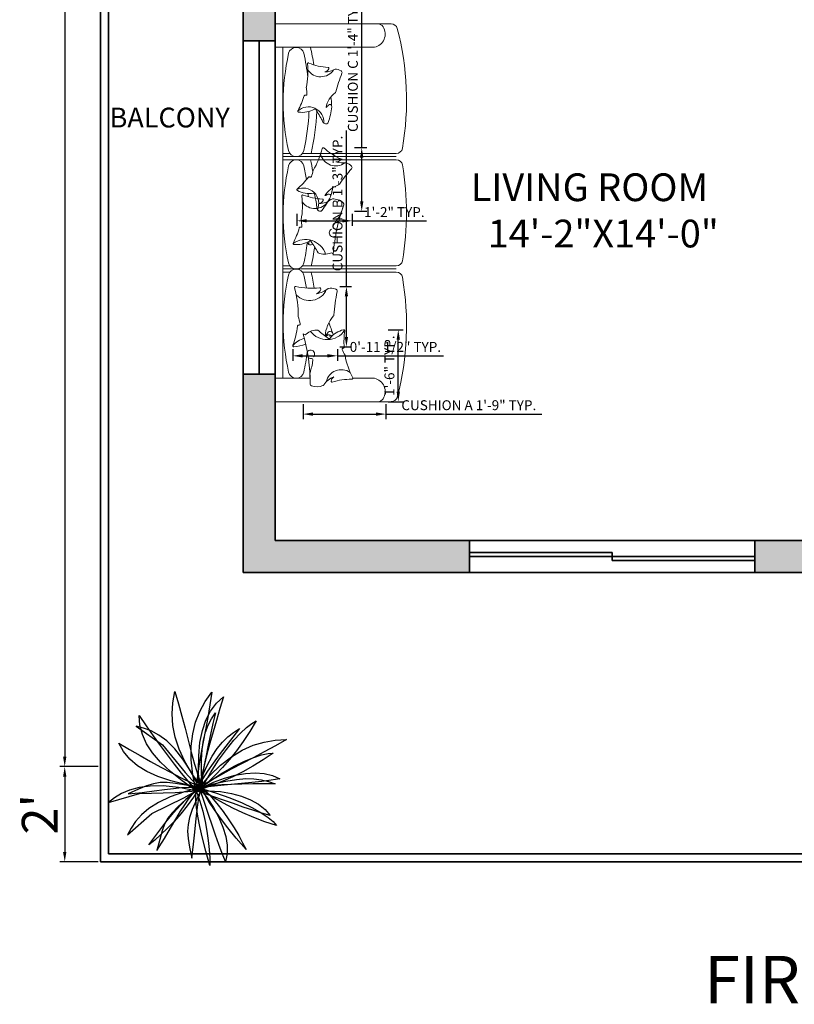
# Model space of a CAD drawing. Units: inches. Extents: x 1566 to 2546, y 1087 to 2705.
# Tile 12 of 27: x 2042 to 2237, y 1100 to 1349. Entities that reach past the tile are written whole.
import ezdxf

# ---------------------------------------------------------------- set-up
doc = ezdxf.new("R2010")
doc.units = ezdxf.units.IN
for name, color, linetype, lineweight in [('A-ANNO-DIMS', 2, 'Continuous', 18), ('A-AREA-IDEN', 7, 'Continuous', 18), ('A-FURN', 8, 'Continuous', 18), ('A-WALL', 7, 'Continuous', 35), ('A-WALL-PATT', 8, 'Continuous', 13), ('L-PLNT', 94, 'Continuous', 18)]:
    doc.layers.add(name, color=color, linetype=linetype, lineweight=lineweight)
doc.layers.add('DIENHOA', color=3, linetype='Continuous')
doc.styles.get("Standard").update_dxf_attribs({"font": 'arial.ttf'})
doc.dimstyles.new('ISO-25', dxfattribs={"dimtxt": 2.5, "dimasz": 2.5, "dimexe": 1.25, "dimexo": 0.625, "dimtad": 1, "dimtxsty": 'Standard', "dimcen": 2.5, "dimadec": 0, "dimazin": 0, "dimtfac": 1, "dimtmove": 0, "dimatfit": 3, "dimfxl": 1, "dimarcsym": 0})

# ---------------------------------------------------------------- blocks, each defined once
blk = doc.blocks.new('*D3')
at = {"layer": 'A-ANNO-DIMS', "color": 0, "lineweight": -2, "transparency": 16777216}
for p, q in [((2061.66, 1784.43), (2052.02, 1784.43)), ((2053.27, 1781.93), (2053.27, 1162.93)), ((2061.66, 1160.43), (2052.02, 1160.43))]:
    blk.add_line(p, q, dxfattribs=at)
at = {"layer": 'A-ANNO-DIMS', "color": 0, "transparency": 16777216}
for points in [[(2052.85, 1781.93), (2053.69, 1781.93), (2053.27, 1784.43)], [(2052.85, 1162.93), (2053.69, 1162.93), (2053.27, 1160.43)]]:
    blk.add_solid(points, dxfattribs=at)
at = {"layer": 'Defpoints', "color": 0, "transparency": 16777216}
for p in [(2062.29, 1784.43), (2053.27, 1160.43), (2062.29, 1160.43)]:
    blk.add_point(p, dxfattribs=at)
at = {"layer": 'A-ANNO-DIMS', "color": 0, "transparency": 16777216, "insert": (2048.05, 1472.43), "char_height": 9, "attachment_point": 5, "rotation": 90}
blk.add_mtext("52'", dxfattribs=at)
blk = doc.blocks.new('*D4')
at = {"layer": 'A-ANNO-DIMS', "color": 0, "lineweight": -2, "transparency": 16777216}
for p, q in [((2061.66, 1160.43), (2052.02, 1160.43)), ((2053.27, 1157.93), (2053.27, 1138.93)), ((2061.66, 1136.43), (2052.02, 1136.43))]:
    blk.add_line(p, q, dxfattribs=at)
at = {"layer": 'A-ANNO-DIMS', "color": 0, "transparency": 16777216}
for points in [[(2052.85, 1157.93), (2053.69, 1157.93), (2053.27, 1160.43)], [(2052.85, 1138.93), (2053.69, 1138.93), (2053.27, 1136.43)]]:
    blk.add_solid(points, dxfattribs=at)
at = {"layer": 'Defpoints', "color": 0, "transparency": 16777216}
for p in [(2062.29, 1160.43), (2053.27, 1136.43), (2062.29, 1136.43)]:
    blk.add_point(p, dxfattribs=at)
at = {"layer": 'A-ANNO-DIMS', "color": 0, "transparency": 16777216, "insert": (2048.13, 1148.43), "char_height": 9, "attachment_point": 5, "rotation": 90}
blk.add_mtext("2'", dxfattribs=at)
blk = doc.blocks.new('Cay03_mb')
at = {"layer": 'DIENHOA'}
for p, q in [((118.6, 555.3), (166.2, 599.1)), ((166.2, 599.1), (142.2, 519.4)), ((79.5, 503.7), (118.6, 555.3)), ((48.6, 443.6), (79.5, 503.7)), ((142.2, 519.4), (119, 441.7)), ((-365.2, 390.3), (-414.4, 402.8)), ((-414.4, 402.8), (-240.2, 277.8)), ((25.5, 374.3), (48.6, 443.6)), ((119, 441.7), (96.7, 365.6)), ((-314.9, 371.3), (-365.2, 390.3)), ((-263.5, 343.5), (-314.9, 371.3)), ((-211.2, 304.6), (-263.5, 343.5)), ((9.9, 295.3), (25.5, 374.3)), ((96.7, 365.6), (75.6, 290.6)), ((-240.2, 277.8), (-88.4, 94.9)), ((-158, 252.3), (-211.2, 304.6)), ((1.6, 205.7), (9.9, 295.3)), ((75.6, 290.6), (55.7, 216.3)), ((290.6, 243.2), (363.4, 275.4)), ((363.4, 275.4), (436.8, 297.2)), ((436.8, 297.2), (511, 309.6)), ((511.8, 271.4), (437.6, 231.5)), ((511, 309.6), (585.9, 313.5)), ((585.9, 313.5), (511.8, 271.4)), ((-104.2, 184.4), (-158, 252.3)), ((0.2, 104.9), (1.6, 205.7)), ((55.7, 216.3), (37.3, 142.1)), ((147, 144.1), (218.5, 199.8)), ((218.5, 199.8), (290.6, 243.2)), ((437.6, 231.5), (363.7, 192.9)), ((-49.6, 98.5), (-104.2, 184.4)), ((37.3, 142.1), (20.5, 67.6)), ((75.9, 75.2), (147, 144.1)), ((290.2, 154.9), (217.4, 116.6)), ((363.7, 192.9), (290.2, 154.9)), ((-88.4, 94.9), (5.4, -7.8)), ((5.4, -7.8), (-49.6, 98.5)), ((5.4, -7.8), (0.2, 104.9)), ((5.4, -7.8), (75.9, 75.2)), ((20.5, 67.6), (5.4, -7.8)), ((145.5, 77.3), (74.7, 36.1)), ((217.4, 116.6), (145.5, 77.3)), ((-345, 5.4), (-399.6, -17.1)), ((-298.6, 20.1), (-345, 5.4)), ((-254.7, 27.4), (-298.6, 20.1)), ((-208, 27.8), (-254.7, 27.4)), ((-152.7, 21.7), (-208, 27.8)), ((-83.4, 9.7), (-152.7, 21.7)), ((5.4, -7.8), (-83.4, 9.7)), ((74.7, 36.1), (5.4, -7.8)), ((5.4, -7.8), (100.3, 18.4)), ((46.3, 0.9), (5.4, -7.8)), ((96.7, 7.5), (46.3, 0.9)), ((155, 12.2), (96.7, 7.5)), ((100.3, 18.4), (182.2, 37.2)), ((219.6, 15.4), (155, 12.2)), ((182.2, 37.2), (253, 48.9)), ((289, 17.4), (219.6, 15.4)), ((253, 48.9), (314.6, 54.1)), ((361.6, 18.5), (289, 17.4)), ((314.6, 54.1), (369.2, 53.3)), ((435.8, 18.9), (361.6, 18.5)), ((369.2, 53.3), (418.6, 46.8)), ((418.6, 46.8), (464.9, 35.2)), ((510, 19), (435.8, 18.9)), ((464.9, 35.2), (510, 19)), ((-399.6, -17.1), (-468, -47.9)), ((-468, -47.9), (-375.6, -37.8)), ((-375.6, -37.8), (-295.3, -27.9)), ((-295.3, -27.9), (-225.8, -18.9)), ((-225.8, -18.9), (-165.8, -11.3)), ((-165.8, -11.3), (-114, -5.7)), ((-114, -5.7), (-69, -2.9)), ((-79.8, -79.6), (-45.1, -46.3)), ((-69, -2.9), (-29.6, -3.4)), ((-45.1, -46.3), (-16.5, -22.4)), ((5.4, -7.8), (-33.2, -69.5)), ((-29.6, -3.4), (5.4, -7.8)), ((-16.5, -22.4), (5.4, -7.8)), ((5.4, -7.8), (56.8, -73.3)), ((25.9, -64.4), (5.4, -7.8)), ((5.4, -7.8), (112.8, -40.3)), ((53.5, -41.6), (5.4, -7.8)), ((47, -125.9), (25.9, -64.4)), ((107, -75.7), (53.5, -41.6)), ((112.8, -40.3), (207.5, -73.8)), ((-165.9, -174.1), (-120.2, -122.1)), ((-120.2, -122.1), (-79.8, -79.6)), ((-74.6, -127.3), (-117.8, -181.1)), ((-33.2, -69.5), (-74.6, -127.3)), ((68.7, -190.6), (47, -125.9)), ((56.8, -73.3), (100.4, -139.1)), ((165.5, -109.6), (107, -75.7)), ((228.7, -142.8), (165.5, -109.6)), ((207.5, -73.8), (289.5, -107.6)), ((289.5, -107.6), (359.3, -141.1)), ((-216.3, -235.6), (-165.9, -174.1)), ((-117.8, -181.1), (-162.1, -230.9)), ((90.8, -256.6), (68.7, -190.6)), ((100.4, -139.1), (135.9, -204.3)), ((296, -174.7), (228.7, -142.8)), ((367.1, -204.8), (296, -174.7)), ((359.3, -141.1), (416.9, -173.5)), ((416.9, -173.5), (462.6, -204.2)), ((-271, -306.6), (-216.3, -235.6)), ((-162.1, -230.9), (-206.3, -276.5)), ((113.1, -322.2), (90.8, -256.6)), ((135.9, -204.3), (162.8, -268.3)), ((441.6, -232.7), (367.1, -204.8)), ((518.9, -257.7), (441.6, -232.7)), ((462.6, -204.2), (496.5, -232.5)), ((496.5, -232.5), (518.9, -257.7)), ((-329.5, -387.1), (-271, -306.6)), ((-249.6, -317.8), (-291, -354.7)), ((-206.3, -276.5), (-249.6, -317.8)), ((135.4, -385.6), (113.1, -322.2)), ((162.8, -268.3), (181, -330.4)), ((-291, -354.7), (-329.5, -387.1)), ((157.6, -445), (135.4, -385.6)), ((181, -330.4), (190, -390)), ((190, -390), (189.6, -446.3)), ((179.5, -498.7), (157.6, -445)), ((189.6, -446.3), (179.5, -498.7))]:
    blk.add_line(p, q, dxfattribs=at)
for points in [[(23.7, -5.4), (-41, 82.2), (-91.8, 167.1), (-129.7, 249.5), (-155.6, 329.6), (-170.2, 407.8), (-174.7, 484.2), (-169.8, 559.3), (-156.5, 633.1)], [(-156.5, 633.1), (-132.5, 551.3), (-110.5, 470), (-89.8, 389.2), (-69.6, 309), (-49, 229.4), (-27.1, 150.4), (-3.2, 72.1), (23.7, -5.4)], [(-16.4, -26.7), (-38.3, 80), (-48.9, 178.3), (-48.7, 269), (-38.5, 352.6), (-19.1, 429.7), (9, 501), (44.9, 567.1), (87.9, 628.5)], [(87.9, 628.5), (75.5, 544.2), (61.3, 461.2), (46.1, 379.1), (30.8, 297.8), (16.1, 216.9), (2.9, 136), (-8.3, 54.9), (-16.4, -26.7)], [(-395.6, 473.7), (-347.5, 405.6), (-300.6, 339.5), (-254.3, 275.1), (-208.3, 212.3), (-161.9, 150.9), (-114.8, 90.7), (-66.5, 31.6), (-16.4, -26.7)], [(-16.4, -26.7), (-108.3, 38.6), (-186.9, 101.7), (-252.4, 163.5), (-305.1, 224.4), (-345.4, 285.2), (-373.7, 346.6), (-390.4, 409.2), (-395.6, 473.7)], [(23.7, -5.4), (19.8, 93), (20.3, 177), (25, 248.5), (34, 309.8), (47.3, 362.7), (64.9, 409.3), (86.8, 451.7), (112.9, 491.9)], [(112.9, 491.9), (96, 419.7), (79.5, 347.4), (63.9, 276.5), (50, 208.4), (38.4, 144.8), (29.7, 86.9), (24.6, 36.3), (23.7, -5.4)], [(384.3, 437.5), (342.2, 367.8), (298.1, 301.7), (252.6, 239.4), (206.1, 181.1), (159.4, 127.2), (113, 78), (67.6, 33.6), (23.7, -5.4)], [(23.7, -5.4), (79.9, 91.7), (134.1, 176.2), (185.8, 248.4), (234.3, 308.7), (279, 357.3), (319.3, 394.8), (354.6, 421.4), (384.3, 437.5)], [(273.2, 387.3), (227.6, 328.8), (182.3, 270.1), (138.4, 212.3), (97.2, 156.4), (60, 103.4), (27.8, 54.6), (1.9, 10.8), (-16.4, -26.7)], [(-16.4, -26.7), (21.4, 64.2), (57, 140.3), (91.4, 203.3), (125.2, 255.1), (159.5, 297.5), (195, 332.5), (232.7, 361.8), (273.2, 387.3)], [(-530.5, 289.7), (-458.3, 248.1), (-387.9, 207.8), (-318.9, 168.7), (-250.8, 131.1), (-182.9, 94.8), (-114.9, 59.9), (-46.2, 26.5), (23.7, -5.4)], [(23.7, -5.4), (-87.2, 15.2), (-185, 39.6), (-270.3, 68.2), (-343.7, 101.4), (-405.9, 139.7), (-457.3, 183.5), (-498.7, 233.4), (-530.5, 289.7)], [(496.7, 224), (429.4, 178.4), (361.6, 136.9), (294.1, 99.5), (227.5, 66.1), (162.4, 36.7), (99.7, 11.5), (39.8, -9.7), (-16.4, -26.7)], [(-16.4, -26.7), (75.4, 37.9), (160.1, 91.8), (237.3, 135.7), (306.6, 170), (367.6, 195.4), (419.9, 212.5), (463.1, 221.9), (496.7, 224)], [(23.7, -5.4), (99.3, 29.7), (173.2, 57.1), (244.8, 76.7), (313.3, 88.3), (377.9, 91.8), (437.9, 87), (492.7, 73.8), (541.4, 52)], [(-16.4, -26.7), (-134, -4.7), (-235.3, 5.3), (-322, 4.7), (-395.9, -5), (-458.7, -22.3), (-512.3, -45.7), (-558.2, -73.6), (-598.4, -104.7)], [(541.4, 52), (484.1, 42.9), (421.2, 34.8), (354.4, 27.6), (285.4, 20.9), (216.1, 14.5), (148.2, 8.1), (83.5, 1.6), (23.7, -5.4)], [(-598.4, -104.7), (-392.7, -44.4), (-155, -37.4), (-16.4, -26.7)], [(-471.9, -320.3), (-310.5, -179.3), (-97.7, -73.3), (23.7, -5.4)], [(23.7, -5.4), (-92.3, -34.8), (-188.4, -68.2), (-266.9, -105.1), (-329.9, -144.9), (-379.7, -187), (-418.5, -230.7), (-448.5, -275.3), (-471.9, -320.3)], [(-276.2, -424.4), (-227.3, -345.4), (-185.7, -276.1), (-150, -215.7), (-119.1, -163.8), (-91.5, -119.5), (-66, -82.3), (-41.4, -51.6), (-16.4, -26.7)], [(-16.4, -26.7), (-84.9, -86), (-137, -133.1), (-175.8, -173), (-204.3, -210), (-225.5, -249.1), (-242.5, -294.7), (-258.4, -351.6), (-276.2, -424.4)], [(23.7, -5.4), (-13.6, -87.9), (-41.1, -152.6), (-59.6, -205), (-69.9, -250.7), (-72.8, -295), (-69.2, -343.6), (-59.7, -401.9), (-45.3, -475.5)], [(-45.3, -475.5), (-34.1, -383.2), (-25.4, -302.8), (-18.3, -233.1), (-12, -172.9), (-5.6, -121.2), (2, -76.8), (11.4, -38.5), (23.7, -5.4)], [(76.2, -524.2), (48.8, -428.5), (26.6, -341.7), (9.2, -264.1), (-3.6, -196.1), (-12.3, -138), (-17.1, -90.2), (-18.3, -53), (-16.4, -26.7)], [(-16.4, -26.7), (66.9, -26.6), (145.6, -32.7), (218.8, -44.9), (285.8, -63.1), (345.9, -87.1), (398.4, -116.6), (442.6, -151.6), (477.6, -191.8)], [(477.6, -191.8), (421.8, -176), (361.3, -156.9), (297.6, -135.5), (232.2, -112.6), (166.6, -89.4), (102.3, -66.6), (40.8, -45.4), (-16.4, -26.7)], [(-16.4, -26.7), (8.5, -95.1), (28.5, -163.3), (44.3, -230.6), (56.3, -296.1), (65, -359), (70.9, -418.5), (74.5, -473.9), (76.2, -524.2)], [(316.5, -418.1), (251.4, -342.8), (194.8, -273.3), (146.5, -210.2), (106.3, -153.8), (74.1, -104.7), (49.7, -63.4), (32.9, -30.1), (23.7, -5.4)], [(23.7, -5.4), (74.9, -57.1), (121.8, -110.6), (164.3, -165), (202.7, -219.4), (237, -272.9), (267.3, -324.5), (293.7, -373.2), (316.5, -418.1)]]:
    blk.add_lwpolyline(points, dxfattribs=at)
blk = doc.blocks.new('CUSHION-A')
blk.add_line((12.54, 5.91), (18.02, 5.91))
for centre, radius, start, end in [((3.38, 14.21), 3.83, 84.2387, 132.8337), ((6.08, 20.97), 5.32, 217.6048, 326.1053), ((33.69, 53.65), 46.53, 229.9755, 234.1671), ((11.64, 12), 6.29, 102.876, 140.0789), ((10.29, 17.91), 0.236, 351.7886, 102.876), ((10.29, 17.91), 0.236, 351.7886, 102.876), ((30.09, 15.05), 19.77, 171.7886, 183.7804), ((0.45, 17.36), 0.472, 195.6578, 312.8337), ((-47.31, 3.98), 49.13, 0.5535, 15.4148), ((6.59, 16.12), 0.236, 234.1671, 341.1685), ((-41.81, -4.21), 52.85, 22.7112, 23.5018), ((10.12, 13.26), 0.236, 89.311, 200.6915), ((18.72, 16.51), 9.43, 200.6915, 210.5832), ((10.12, 13.73), 0.236, 269.311, 3.7804), ((1.93, 11.97), 1.05, 232.8444, 267.2985), ((-19.11, 13.83), 21.87, 342.6177, 350.951), ((1.9, 11.4), 0.472, 267.2985, 277.3574), ((2.02, 10.46), 0.472, 350.951, 97.3574), ((30.09, 15.05), 19.77, 189.7298, 207.2752), ((2.2, 7.1), 0.472, 156.2045, 183.614), ((-47.31, 3.98), 49.13, 0.5535, 3.614), ((9.43, 1.66), 4.91, 110.2155, 148.3929), ((7.3, 5.16), 0.236, 171.7015, 287.2637), ((8.61, 4.97), 1.56, 124.2109, 171.7015), ((12.04, -10.09), 15.74, 89.041, 107.2637), ((12.31, 5.88), 0.236, 269.041, 27.2752), ((17.28, 2.55), 3.44, 328.6411, 77.5888), ((2.29, 4.45), 0.472, 180.5535, 248.334), ((3.54, 7.6), 3.85, 248.334, 292.6623), ((4.84, 4.48), 0.472, 292.6623, 328.3929), ((18.88, 1.57), 1.57, 270, 328.6411)]:
    blk.add_arc(centre, radius, start, end)
blk = doc.blocks.new('CUSHION-B')
for centre, radius, start, end in [((0.72, 14.91), 0.283, 77.7826, 196.0168), ((4.78, 33.64), 18.88, 257.7826, 276.0053), ((-22.35, 8.29), 23.73, 358.4714, 16.0168), ((5.1, 19.21), 5.89, 278.9571, 310.4913), ((5.29, 15.11), 1.87, 292.9525, 340.443), ((6.79, 14.58), 0.283, 340.443, 96.0053), ((9.49, 10.31), 4.45, 72.8696, 97.2038), ((69.07, 2.72), 58.96, 169.0518, 174.8479), ((10.63, 14.03), 0.567, 349.0518, 72.8696), ((-9.32, 3.91), 11.32, 9.4331, 19.3248), ((16.33, 2.29), 8.16, 138.6039, 177.0681), ((9.79, 8.07), 0.567, 317.5655, 354.8479), ((-22.35, 8.29), 23.73, 340.5302, 352.522), ((1.45, 5.16), 0.283, 78.0525, 172.522), ((1.57, 5.72), 0.283, 258.0525, 9.4331), ((2.15, 7.87), 7.94, 319.38, 328.0577), ((9.14, 2.07), 0.945, 40.8427, 147.338), ((9.41, 3.05), 0.814, 43.9174, 130.1627), ((0.28, 0.28), 0.283, 160.5302, 271.6176), ((3.81, -2.51), 4.68, 100.8696, 144.3073), ((0.08, 7.55), 7.55, 271.6176, 294.8398)]:
    blk.add_arc(centre, radius, start, end)
blk = doc.blocks.new('CUSHION-C')
for centre, radius, start, end in [((-12.77, 20.63), 19.77, 328.4714, 346.0168), ((6.65, 15.79), 0.236, 47.7826, 166.0168), ((17.38, 27.62), 15.74, 227.7826, 246.0053), ((10.03, 14.04), 1.56, 262.9525, 310.443), ((11.6, 17.07), 4.91, 248.9571, 280.4913), ((10.89, 13.03), 0.236, 310.443, 66.0053), ((-5.18, 12.04), 9.43, 339.4331, 349.3248), ((50.9, -21.48), 49.13, 139.0518, 144.8479), ((11.06, 8.82), 3.71, 42.8696, 67.2038), ((13.43, 11.03), 0.472, 319.0518, 42.8696), ((-12.77, 20.63), 19.77, 310.5302, 322.522), ((3.11, 8.45), 0.236, 48.0525, 142.522), ((3.43, 8.81), 0.236, 228.0525, 339.4331), ((0.24, 5.42), 0.236, 130.5302, 241.6176), ((1.61, 1.94), 3.9, 336.4825, 114.3073), ((3.12, 10.75), 6.29, 241.6176, 279.5758), ((12.33, 0.78), 6.13, 107.5655, 149.079), ((10.34, 7.08), 0.472, 287.5655, 324.8479), ((4.2, 4.31), 0.236, 12.8897, 99.5758), ((-40.92, -6.02), 46.53, 8.8632, 12.8897), ((-7.53, 11.48), 17.84, 320.6607, 333.8744), ((5.34, 8.91), 5.27, 289.1869, 298.5341), ((8.08, 3.87), 0.472, 329.5475, 118.5341), ((5.93, 0.92), 0.917, 164.9476, 266.1991), ((5.9, 0.47), 0.472, 266.1991, 320.6607)]:
    blk.add_arc(centre, radius, start, end)
blk = doc.blocks.new('*D51')
at = {"layer": 'A-ANNO-DIMS', "color": 0, "lineweight": -2, "transparency": 16777216}
for p, q in [((2113.35, 1251.84), (2113.35, 1248.08)), ((2134.23, 1251.84), (2134.23, 1248.08)), ((2115.85, 1249.33), (2131.73, 1249.33)), ((2134.23, 1249.33), (2173.57, 1249.33))]:
    blk.add_line(p, q, dxfattribs=at)
at = {"layer": 'A-ANNO-DIMS', "color": 0, "transparency": 16777216}
for points in [[(2115.85, 1249.75), (2115.85, 1248.91), (2113.35, 1249.33)], [(2131.73, 1249.75), (2131.73, 1248.91), (2134.23, 1249.33)]]:
    blk.add_solid(points, dxfattribs=at)
at = {"layer": 'Defpoints', "color": 0, "transparency": 16777216}
for p in [(2113.35, 1252.46), (2134.23, 1252.46), (2134.23, 1249.33)]:
    blk.add_point(p, dxfattribs=at)
at = {"layer": 'A-ANNO-DIMS', "color": 0, "transparency": 16777216, "insert": (2155.15, 1251.25), "char_height": 2.5, "attachment_point": 5}
blk.add_mtext('CUSHION A 1\'-9" TYP.', dxfattribs=at)
blk = doc.blocks.new('*D52')
at = {"layer": 'A-ANNO-DIMS', "color": 0, "lineweight": -2, "transparency": 16777216}
for p, q in [((2134.86, 1270.62), (2138.62, 1270.62)), ((2137.37, 1254.96), (2137.37, 1268.12)), ((2134.86, 1252.46), (2138.62, 1252.46))]:
    blk.add_line(p, q, dxfattribs=at)
at = {"layer": 'A-ANNO-DIMS', "color": 0, "transparency": 16777216}
for points in [[(2136.95, 1268.12), (2137.78, 1268.12), (2137.37, 1270.62)], [(2136.95, 1254.96), (2137.78, 1254.96), (2137.37, 1252.46)]]:
    blk.add_solid(points, dxfattribs=at)
at = {"layer": 'Defpoints', "color": 0, "transparency": 16777216}
for p in [(2134.23, 1270.62), (2137.37, 1270.62), (2134.23, 1252.46)]:
    blk.add_point(p, dxfattribs=at)
at = {"layer": 'A-ANNO-DIMS', "color": 0, "transparency": 16777216, "insert": (2135.46, 1261.54), "char_height": 2.5, "attachment_point": 5, "rotation": 90}
blk.add_mtext('1\'-6" TYP.', dxfattribs=at)
blk = doc.blocks.new('*D53')
at = {"layer": 'A-ANNO-DIMS', "color": 0, "lineweight": -2, "transparency": 16777216}
for p, q in [((2124.29, 1281.52), (2124.29, 1320.86)), ((2122.64, 1281.52), (2125.54, 1281.52)), ((2124.29, 1268.81), (2124.29, 1279.02)), ((2122.64, 1266.31), (2125.54, 1266.31))]:
    blk.add_line(p, q, dxfattribs=at)
at = {"layer": 'A-ANNO-DIMS', "color": 0, "transparency": 16777216}
for points in [[(2123.88, 1279.02), (2124.71, 1279.02), (2124.29, 1281.52)], [(2123.88, 1268.81), (2124.71, 1268.81), (2124.29, 1266.31)]]:
    blk.add_solid(points, dxfattribs=at)
at = {"layer": 'Defpoints', "color": 0, "transparency": 16777216}
for p in [(2122.01, 1281.52), (2124.29, 1281.52), (2122.01, 1266.31)]:
    blk.add_point(p, dxfattribs=at)
at = {"layer": 'A-ANNO-DIMS', "color": 0, "transparency": 16777216, "insert": (2122.37, 1302.44), "char_height": 2.5, "attachment_point": 5, "rotation": 90}
blk.add_mtext('CUSHION B 1\'-3" TYP.', dxfattribs=at)
blk = doc.blocks.new('*D54')
at = {"layer": 'A-ANNO-DIMS', "color": 0, "lineweight": -2, "transparency": 16777216}
for p, q in [((2110.75, 1265.69), (2110.75, 1262.78)), ((2113.25, 1264.03), (2119.51, 1264.03)), ((2122.01, 1265.69), (2122.01, 1262.78)), ((2122.01, 1264.03), (2148.77, 1264.03))]:
    blk.add_line(p, q, dxfattribs=at)
at = {"layer": 'A-ANNO-DIMS', "color": 0, "transparency": 16777216}
for points in [[(2113.25, 1264.45), (2113.25, 1263.61), (2110.75, 1264.03)], [(2119.51, 1264.45), (2119.51, 1263.61), (2122.01, 1264.03)]]:
    blk.add_solid(points, dxfattribs=at)
at = {"layer": 'Defpoints', "color": 0, "transparency": 16777216}
for p in [(2110.75, 1266.31), (2122.01, 1266.31), (2122.01, 1264.03)]:
    blk.add_point(p, dxfattribs=at)
at = {"layer": 'A-ANNO-DIMS', "color": 0, "transparency": 16777216, "insert": (2136.64, 1265.95), "char_height": 2.5, "attachment_point": 5}
blk.add_mtext('0\'-11 1/2" TYP.', dxfattribs=at)
blk = doc.blocks.new('*D55')
at = {"layer": 'A-ANNO-DIMS', "color": 0, "lineweight": -2, "transparency": 16777216}
for p, q in [((2128.15, 1316.53), (2128.15, 1356.06)), ((2126.37, 1316.53), (2129.4, 1316.53)), ((2128.15, 1302.98), (2128.15, 1314.03)), ((2126.37, 1300.48), (2129.4, 1300.48))]:
    blk.add_line(p, q, dxfattribs=at)
at = {"layer": 'A-ANNO-DIMS', "color": 0, "transparency": 16777216}
for points in [[(2127.74, 1314.03), (2128.57, 1314.03), (2128.15, 1316.53)], [(2127.74, 1302.98), (2128.57, 1302.98), (2128.15, 1300.48)]]:
    blk.add_solid(points, dxfattribs=at)
at = {"layer": 'Defpoints', "color": 0, "transparency": 16777216}
for p in [(2125.75, 1316.53), (2128.15, 1316.53), (2125.75, 1300.48)]:
    blk.add_point(p, dxfattribs=at)
at = {"layer": 'A-ANNO-DIMS', "color": 0, "transparency": 16777216, "insert": (2126.24, 1337.54), "char_height": 2.5, "attachment_point": 5, "rotation": 90}
blk.add_mtext('CUSHION C 1\'-4" TYP.', dxfattribs=at)
blk = doc.blocks.new('*D56')
at = {"layer": 'A-ANNO-DIMS', "color": 0, "lineweight": -2, "transparency": 16777216}
for p, q in [((2111.8, 1299.85), (2111.8, 1296.82)), ((2125.75, 1299.85), (2125.75, 1296.82)), ((2114.3, 1298.07), (2123.25, 1298.07)), ((2125.75, 1298.07), (2144.5, 1298.07))]:
    blk.add_line(p, q, dxfattribs=at)
at = {"layer": 'A-ANNO-DIMS', "color": 0, "transparency": 16777216}
for points in [[(2114.3, 1298.49), (2114.3, 1297.65), (2111.8, 1298.07)], [(2123.25, 1298.49), (2123.25, 1297.65), (2125.75, 1298.07)]]:
    blk.add_solid(points, dxfattribs=at)
at = {"layer": 'Defpoints', "color": 0, "transparency": 16777216}
for p in [(2111.8, 1300.48), (2125.75, 1300.48), (2125.75, 1298.07)]:
    blk.add_point(p, dxfattribs=at)
at = {"layer": 'A-ANNO-DIMS', "color": 0, "transparency": 16777216, "insert": (2136.37, 1299.95), "char_height": 2.5, "attachment_point": 5}
blk.add_mtext('1\'-2" TYP.', dxfattribs=at)

msp = doc.modelspace()

# ---------------------------------------------------------------- hatches: boundary and pattern name
at = {"layer": 'A-WALL-PATT'}
h = msp.add_hatch(color=256, dxfattribs=at)
h.dxf.hatch_style = 1
h.paths.add_polyline_path([(2106.29, 1385.43), (2228.29, 1385.43), (2228.29, 1391.43), (2224.29, 1391.43), (2224.29, 1389.43), (2106.29, 1389.43), (2106.29, 1402.93), (2098.29, 1402.93), (2098.29, 1343.43), (2106.29, 1343.43), (2106.29, 1347.74)], flags=17)
h.paths.add_polyline_path([(2106.29, 1259.43), (2098.29, 1259.43), (2098.29, 1209.43), (2155.29, 1209.43), (2155.29, 1217.43), (2143.41, 1217.43), (2106.29, 1217.43)], flags=17)
h.paths.add_polyline_path([(2334.29, 1217.43), (2280.29, 1217.43), (2280.29, 1389.43), (2284.29, 1389.43), (2284.29, 1391.43), (2284.29, 1393.43), (2276.29, 1393.43), (2276.29, 1217.43), (2227.29, 1217.43), (2227.29, 1209.43), (2334.29, 1209.43)], flags=17)
h.paths.add_polyline_path([(2106.29, 1486.43), (2098.29, 1486.43), (2098.29, 1460.88), (2099.11, 1461.64), (2100.44, 1462.65), (2101.57, 1463.26), (2099.97, 1460.62), (2098.29, 1458.1), (2098.29, 1456.93), (2100.35, 1456.93), (2100.77, 1457.12), (2103.56, 1457.95), (2106.29, 1458.4), (2106.29, 1470.43), (2224.29, 1470.43), (2224.29, 1427.43), (2228.29, 1427.43), (2228.29, 1474.43), (2192.29, 1474.43), (2192.29, 1476.43), (2188.29, 1476.43), (2188.29, 1474.43), (2106.29, 1474.43)], flags=17)
h.paths.add_polyline_path([(2106.29, 1585.43), (2192.29, 1585.43), (2192.29, 1589.43), (2098.29, 1589.43), (2098.29, 1573.93), (2106.29, 1573.93)], flags=17)
h.paths.add_polyline_path([(2228.29, 1585.43), (2232.29, 1585.43), (2232.29, 1589.43), (2224.29, 1589.43), (2222.29, 1589.43), (2222.29, 1585.43), (2224.29, 1585.43), (2224.29, 1532.43), (2106.29, 1532.43), (2106.29, 1543.93), (2098.29, 1543.93), (2098.29, 1516.43), (2106.29, 1516.43), (2106.29, 1528.43), (2188.29, 1528.43), (2188.29, 1506.43), (2192.29, 1506.43), (2192.29, 1528.43), (2224.29, 1528.43), (2224.29, 1506.43), (2228.29, 1506.43)], flags=17)
h.paths.add_polyline_path([(2106.29, 1680.43), (2098.29, 1680.43), (2098.29, 1625.43), (2106.29, 1625.43)], flags=17)
h.paths.add_polyline_path([(2458.29, 1784.43), (2098.29, 1784.43), (2098.29, 1776.43), (2276.29, 1776.43), (2276.29, 1589.43), (2268.29, 1589.43), (2268.29, 1585.43), (2280.29, 1585.43), (2280.29, 1652.43), (2284.29, 1652.43), (2284.29, 1656.43), (2280.29, 1656.43), (2280.29, 1776.43), (2398.29, 1776.43), (2398.29, 1746.43), (2402.29, 1746.43), (2402.29, 1776.43), (2450.29, 1776.43), (2450.29, 1532.43), (2375.49, 1532.43), (2328.29, 1532.43), (2328.29, 1612.43), (2324.29, 1612.43), (2324.29, 1528.43), (2450.29, 1528.43), (2450.29, 1447.43), (2291.29, 1447.43), (2291.29, 1443.43), (2324.29, 1443.43), (2324.29, 1393.43), (2320.29, 1393.43), (2320.29, 1389.43), (2330.29, 1389.43), (2330.29, 1393.43), (2328.29, 1393.43), (2328.29, 1443.43), (2412.29, 1443.43), (2412.29, 1433.43), (2416.29, 1433.43), (2416.29, 1443.43), (2450.29, 1443.43), (2450.29, 1393.43), (2416.29, 1393.43), (2416.29, 1403.43), (2412.29, 1403.43), (2412.29, 1393.43), (2360.29, 1393.43), (2360.29, 1389.43), (2450.29, 1389.43), (2450.29, 1217.43), (2396.29, 1217.43), (2396.29, 1209.43), (2450.29, 1209.43), (2450.29, 1136.43), (2458.29, 1136.43)])

# ---------------------------------------------------------------- linework, layer by layer
at = {"layer": 'A-FURN'}
for p, q in [((2106.29, 1252.46), (2106.29, 1347.74)), ((2106.29, 1347.74), (2135.58, 1347.74)), ((2106.29, 1341.83), (2131.37, 1341.83)), ((2108.26, 1258.37), (2108.26, 1341.83)), ((2108.26, 1315.06), (2110.02, 1315.06)), ((2108.26, 1314.27), (2136.87, 1314.27)), ((2108.26, 1313.49), (2136.87, 1313.49)), ((2113.24, 1315.06), (2136.87, 1315.06)), ((2108.26, 1286.71), (2110.02, 1286.71)), ((2113.24, 1286.71), (2136.87, 1286.71)), ((2108.26, 1285.93), (2136.87, 1285.93)), ((2108.26, 1285.14), (2110.02, 1285.14)), ((2113.24, 1285.14), (2136.87, 1285.14)), ((2106.29, 1258.37), (2115.13, 1258.37)), ((2106.29, 1252.46), (2135.58, 1252.46)), ((2219, 1217.43), (2143.41, 1217.43))]:
    msp.add_line(p, q, dxfattribs=at)
for centre, radius, start, end in [((2130.63, 1345.19), 3.44, 282.4112, 31.3589), ((2132.23, 1346.16), 1.57, 31.3589, 90), ((2135.58, 1346.16), 1.57, 14.7607, 90), ((2068.34, 1328.45), 71.11, 350.2206, 14.7607), ((2111.63, 1339.83), 1.97, 14.0803, 165.9197), ((2058.7, 1328.01), 58.17, 9.2978, 13.7486), ((2164.56, 1328.01), 56.2, 167.3591, 192.5496), ((2058.7, 1328.01), 56.2, 6.399, 12.6409), ((2117.81, 1338.32), 3.93, 214.8494, 325.9788), ((2111.1, 1327.36), 9.43, 359.0692, 11.4619), ((2058.7, 1328.01), 56.2, 347.4504, 357.5986), ((2058.7, 1328.01), 58.17, 347.1404, 357.743), ((2136.87, 1316.63), 1.57, 270, 350.2206), ((2111.63, 1316.26), 1.98, 193.4421, 346.5579), ((2058.7, 1299.66), 58.17, 10.7847, 13.7486), ((2121.58, 1315.85), 3.93, 194.8494, 305.9788), ((2136.87, 1311.91), 1.57, 9.7794, 90), ((2164.56, 1299.66), 56.2, 167.3591, 192.5496), ((2111.63, 1311.48), 1.97, 14.0803, 165.9197), ((2058.7, 1299.66), 56.2, 8.9885, 12.6409), ((2068.34, 1300.1), 71.11, 350.2206, 9.7794), ((2111.53, 1307.85), 9.43, 339.0692, 351.4619), ((2093.43, 1301.82), 19.77, 349.7298, 7.2752), ((2113.28, 1304.35), 0.236, 69.041, 187.2752), ((2118.99, 1319.27), 15.74, 249.041, 267.2637), ((2058.7, 1299.66), 56.2, 4.5548, 5.3997), ((2118.23, 1303.32), 0.236, 331.7015, 87.2637), ((2120.77, 1303.12), 0.472, 92.6623, 128.3929), ((2120.93, 1299.75), 3.85, 48.334, 92.6623), ((2116.36, 1305.09), 3.93, 216.1078, 327.2372), ((2117.43, 1307.34), 4.91, 270.2155, 308.3929), ((2117.07, 1303.94), 1.56, 284.2109, 331.7015), ((2169.95, 1285.76), 49.13, 160.5535, 175.4148), ((2169.95, 1285.76), 49.13, 160.5535, 163.614), ((2123.18, 1302.27), 0.472, 340.5535, 48.334), ((2140.08, 1286.14), 21.87, 142.6177, 150.951), ((2122.36, 1299.75), 0.472, 316.2045, 343.614), ((2093.43, 1301.82), 19.77, 331.7886, 343.7804), ((2112.64, 1296.23), 0.236, 69.311, 163.7804), ((2112.81, 1296.67), 0.236, 249.311, 0.6915), ((2103.62, 1296.56), 9.43, 0.6915, 10.5832), ((2121.38, 1296.53), 0.472, 150.951, 257.3574), ((2120.95, 1295.02), 0.999, 114.2238, 307.6435), ((2121.17, 1295.61), 0.472, 67.2985, 77.3574), ((2120.95, 1295.08), 1.05, 32.8444, 67.2985), ((2113.97, 1288.04), 5.32, 17.6048, 126.1053), ((2111.06, 1292.36), 0.236, 151.7886, 262.876), ((2111.06, 1292.36), 0.236, 151.7886, 262.876), ((2111.82, 1298.37), 6.29, 262.876, 300.0789), ((2058.7, 1299.66), 56.2, 347.4504, 352.6454), ((2115.25, 1292.95), 0.945, 200.8427, 307.338), ((2167.59, 1295.33), 52.85, 182.7112, 183.5018), ((2115.15, 1292.78), 0.236, 34.1671, 141.1685), ((2076.85, 1266.78), 46.53, 29.9755, 34.1671), ((2058.7, 1299.66), 58.17, 347.1404, 351.9048), ((2067.37, 1313), 52.85, 337.2794, 337.2982), ((2118.82, 1293.48), 3.83, 244.2387, 292.8337), ((2120.49, 1289.51), 0.472, 355.6578, 112.8337), ((2111.63, 1287.91), 1.98, 193.4421, 346.5579), ((2136.87, 1288.29), 1.57, 270, 350.2206), ((2164.56, 1272.19), 56.2, 167.4504, 192.6409), ((2111.63, 1283.94), 1.98, 13.4421, 166.5579), ((2058.7, 1272.19), 56.2, 9.1435, 12.5496), ((2058.7, 1272.19), 58.17, 8.7934, 12.8596), ((2136.87, 1283.56), 1.57, 9.7794, 90), ((2068.34, 1271.75), 71.11, 345.2393, 9.7794), ((2115.01, 1282.66), 4.71, 224.8494, 335.9788), ((2170.89, 1288.74), 53.54, 197.709, 201.2519), ((2058.7, 1272.19), 56.2, 347.3591, 352.5789), ((2115.26, 1264.49), 0.999, 314.2238, 147.6435), ((2111.63, 1260.37), 1.97, 194.0803, 345.9197), ((2123.02, 1256.6), 3.93, 56.1078, 167.2372), ((2135.58, 1254.04), 1.57, 270, 345.2393)]:
    msp.add_arc(centre, radius, start, end, dxfattribs=at)
at = {"layer": 'A-WALL'}
for p, q in [((2098.29, 1209.43), (2098.29, 1589.43)), ((2062.29, 1474.65), (2062.29, 1136.43)), ((2064.29, 1472.65), (2064.29, 1138.43)), ((2106.29, 1217.43), (2106.29, 1385.43)), ((2106.29, 1343.43), (2098.29, 1343.43)), ((2102.29, 1343.43), (2102.29, 1259.43)), ((2106.29, 1259.43), (2098.29, 1259.43)), ((2106.29, 1217.43), (2276.29, 1217.43)), ((2155.29, 1217.43), (2155.29, 1209.43)), ((2227.29, 1217.43), (2227.29, 1209.43)), ((2155.29, 1214.43), (2191.29, 1214.43)), ((2191.29, 1214.43), (2191.29, 1212.43)), ((2155.29, 1213.43), (2227.29, 1213.43)), ((2191.29, 1212.43), (2227.29, 1212.43)), ((2098.29, 1209.43), (2450.29, 1209.43)), ((2064.29, 1138.43), (2450.29, 1138.43)), ((2062.29, 1136.43), (2458.29, 1136.43))]:
    msp.add_line(p, q, dxfattribs=at)

# ---------------------------------------------------------------- block references
at = {"layer": 'A-FURN', "rotation": 19.99999999998933}
msp.add_blockref('CUSHION-C', (2113.87, 1320.54), dxfattribs=at)
at = {"layer": 'A-FURN'}
for name, p in [('CUSHION-C', (2111.8, 1300.49)), ('CUSHION-B', (2110.77, 1266.31)), ('CUSHION-A', (2113.35, 1252.46))]:
    msp.add_blockref(name, p, dxfattribs=at)
at = {"layer": 'L-PLNT', "xscale": 0.0378941924884598, "yscale": 0.0378941924884598, "zscale": 0.0378941924884598}
msp.add_blockref('Cay03_mb', (2087, 1155.37), dxfattribs=at)

# ---------------------------------------------------------------- texts
at = {"layer": 'A-AREA-IDEN', "attachment_point": 1}
for s, width, insert, char_height in [('BALCONY', 111.7553, (2064.58, 1326.61), 5), ('LIVING ROOM\\P  14\'-2"X14\'-0"', 111.7553, (2155.63, 1310.03), 7), ('FIRST FLOOR PLAN', 179.2212, (2214.47, 1112.71), 12)]:
    msp.add_mtext_dynamic_manual_height_columns(s, width=width, gutter_width=12.5, heights=[0], dxfattribs=dict(at, insert=insert, char_height=char_height))

# ---------------------------------------------------------------- dimensions: what is measured, and where the dimension line sits
at = {"layer": 'A-ANNO-DIMS'}
for base, p1, p2, override, picture, middle in [((2053.27, 1160.43), (2062.29, 1784.43), (2062.29, 1160.43), {"dimtxt": 9, "dimdec": 1, "dimlunit": 3, "dimclrd": 0, "dimclre": 0, "dimclrt": 0, "dimtdec": 1}, '*D3', (2048.05, 1472.43)), ((2053.27, 1136.43), (2062.29, 1160.43), (2062.29, 1136.43), {"dimtxt": 9, "dimdec": 1, "dimlunit": 3, "dimclrd": 0, "dimclre": 0, "dimclrt": 0, "dimtdec": 1, "dimtmove": 1}, '*D4', (2048.13, 1148.43))]:
    dim = msp.add_linear_dim(base=base, p1=p1, p2=p2, angle=90, dimstyle='ISO-25', override=override, dxfattribs=at)
    dim.commit()
    dim.dimension.update_dxf_attribs({"geometry": picture, "text_midpoint": middle})
for base, p1, p2, text, picture, middle in [((2128.1548, 1316.5307), (2125.7469, 1300.4777), (2125.7469, 1316.5307), 'CUSHION C <> TYP.', '*D55', (2126.2364, 1337.5445)), ((2124.29, 1281.52), (2122.01, 1266.31), (2122.01, 1281.52), 'CUSHION B <> TYP.', '*D53', (2122.37, 1302.44)), ((2137.37, 1270.62), (2134.23, 1252.46), (2134.23, 1270.62), '<> TYP.', '*D52', (2135.46, 1261.54))]:
    dim = msp.add_linear_dim(base=base, p1=p1, p2=p2, angle=90, text=text, dimstyle='ISO-25', override={"dimdec": 1, "dimrnd": 0, "dimzin": 1, "dimlunit": 4, "dimfrac": 2}, dxfattribs=at)
    dim.commit()
    dim.dimension.update_dxf_attribs({"geometry": picture, "text_midpoint": middle})
for base, p1, p2, text, picture, middle in [((2125.7469, 1298.0698), (2111.7956, 1300.4777), (2125.7469, 1300.4777), '<> TYP.', '*D56', (2136.3736, 1299.9507)), ((2122.01, 1264.03), (2110.75, 1266.31), (2122.01, 1266.31), '<> TYP.', '*D54', (2136.64, 1265.95)), ((2134.23, 1249.33), (2113.35, 1252.46), (2134.23, 1252.46), 'CUSHION A <> TYP.', '*D51', (2155.15, 1251.25))]:
    dim = msp.add_linear_dim(base=base, p1=p1, p2=p2, text=text, dimstyle='ISO-25', override={"dimdec": 1, "dimrnd": 0, "dimzin": 1, "dimlunit": 4, "dimfrac": 2}, dxfattribs=at)
    dim.commit()
    dim.dimension.update_dxf_attribs({"geometry": picture, "text_midpoint": middle})

doc.saveas('drawing.dxf')
